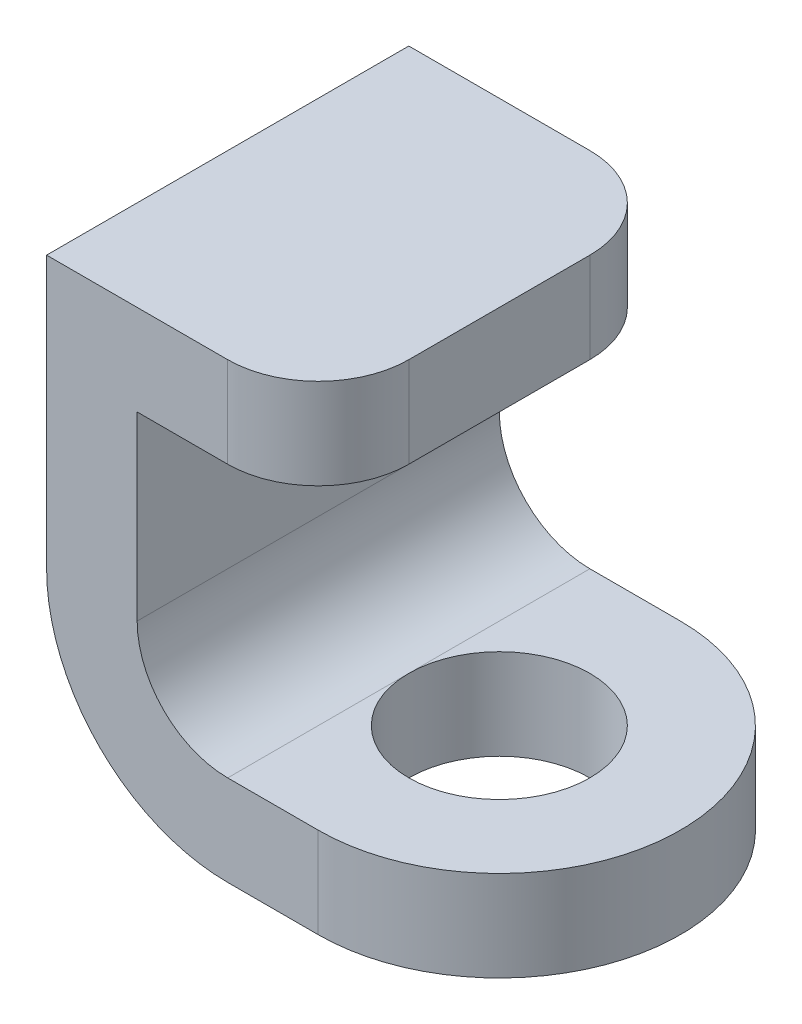
ISO-10303-21;
HEADER;
FILE_DESCRIPTION(('STEP AP214'),'2;1');
FILE_NAME('part.step','',(''),(''),'','','');
FILE_SCHEMA(('AUTOMOTIVE_DESIGN { 1 0 10303 214 1 1 1 1 }'));
ENDSEC;
DATA;
#1=APPLICATION_CONTEXT('core data for automotive mechanical design processes');
#2=APPLICATION_PROTOCOL_DEFINITION('international standard','automotive_design',2000,#1);
#3=PRODUCT_CONTEXT('',#1,'mechanical');
#4=PRODUCT('Part','Part','',(#3));
#5=PRODUCT_RELATED_PRODUCT_CATEGORY('part','',(#4));
#6=PRODUCT_DEFINITION_FORMATION('','',#4);
#7=PRODUCT_DEFINITION_CONTEXT('part definition',#1,'design');
#8=PRODUCT_DEFINITION('design','',#6,#7);
#9=PRODUCT_DEFINITION_SHAPE('','',#8);
#10=(LENGTH_UNIT() NAMED_UNIT(*) SI_UNIT(.MILLI.,.METRE.));
#11=(NAMED_UNIT(*) PLANE_ANGLE_UNIT() SI_UNIT($,.RADIAN.));
#12=(NAMED_UNIT(*) SI_UNIT($,.STERADIAN.) SOLID_ANGLE_UNIT());
#13=UNCERTAINTY_MEASURE_WITH_UNIT(LENGTH_MEASURE(1.E-05),#10,'distance_accuracy_value','');
#14=(GEOMETRIC_REPRESENTATION_CONTEXT(3) GLOBAL_UNCERTAINTY_ASSIGNED_CONTEXT((#13)) GLOBAL_UNIT_ASSIGNED_CONTEXT((#10,
#11,#12)) REPRESENTATION_CONTEXT('',''));
#15=CARTESIAN_POINT('',(0.,0.,0.));
#16=DIRECTION('',(0.,0.,1.));
#17=DIRECTION('',(1.,0.,0.));
#18=AXIS2_PLACEMENT_3D('',#15,#16,#17);
#19=CARTESIAN_POINT('',(50.,0.,20.));
#20=DIRECTION('',(0.,1.,0.));
#21=DIRECTION('',(-1.,0.,0.));
#22=AXIS2_PLACEMENT_3D('',#19,#20,#21);
#23=PLANE('',#22);
#24=DIRECTION('',(0.,0.,-1.));
#25=VECTOR('',#24,1.);
#26=CARTESIAN_POINT('',(20.,0.,20.));
#27=LINE('',#26,#25);
#28=CARTESIAN_POINT('',(20.,0.,20.));
#29=VERTEX_POINT('',#28);
#30=CARTESIAN_POINT('',(20.,0.,0.));
#31=VERTEX_POINT('',#30);
#32=EDGE_CURVE('E215',#29,#31,#27,.T.);
#33=ORIENTED_EDGE('',*,*,#32,.T.);
#34=CARTESIAN_POINT('',(30.,0.,0.));
#35=DIRECTION('',(0.,-1.,0.));
#36=DIRECTION('',(1.,0.,0.));
#37=AXIS2_PLACEMENT_3D('',#34,#35,#36);
#38=CIRCLE('',#37,10.);
#39=EDGE_CURVE('E76',#31,#31,#38,.T.);
#40=ORIENTED_EDGE('',*,*,#39,.F.);
#41=CARTESIAN_POINT('',(20.,0.,-20.));
#42=VERTEX_POINT('',#41);
#43=EDGE_CURVE('E179',#31,#42,#27,.T.);
#44=ORIENTED_EDGE('',*,*,#43,.T.);
#45=DIRECTION('',(1.,0.,0.));
#46=VECTOR('',#45,1.);
#47=CARTESIAN_POINT('',(50.,0.,-20.));
#48=LINE('',#47,#46);
#49=CARTESIAN_POINT('',(30.,0.,-20.));
#50=VERTEX_POINT('',#49);
#51=EDGE_CURVE('E171',#42,#50,#48,.T.);
#52=ORIENTED_EDGE('',*,*,#51,.T.);
#53=CARTESIAN_POINT('',(30.,0.,0.));
#54=DIRECTION('',(0.,-1.,0.));
#55=DIRECTION('',(1.,0.,0.));
#56=AXIS2_PLACEMENT_3D('',#53,#54,#55);
#57=CIRCLE('',#56,20.);
#58=CARTESIAN_POINT('',(30.,0.,20.));
#59=VERTEX_POINT('',#58);
#60=EDGE_CURVE('E154',#50,#59,#57,.T.);
#61=ORIENTED_EDGE('',*,*,#60,.T.);
#62=DIRECTION('',(1.,0.,0.));
#63=VECTOR('',#62,1.);
#64=CARTESIAN_POINT('',(50.,0.,20.));
#65=LINE('',#64,#63);
#66=EDGE_CURVE('E272',#29,#59,#65,.T.);
#67=ORIENTED_EDGE('',*,*,#66,.F.);
#68=EDGE_LOOP('',(#33,#40,#44,#52,#61,#67));
#69=FACE_BOUND('',#68,.T.);
#70=ADVANCED_FACE('F62',(#69),#23,.F.);
#71=CARTESIAN_POINT('',(20.,10.,20.));
#72=DIRECTION('',(0.,-1.,0.));
#73=DIRECTION('',(0.,0.,-1.));
#74=AXIS2_PLACEMENT_3D('',#71,#72,#73);
#75=PLANE('',#74);
#76=DIRECTION('',(0.,0.,-1.));
#77=VECTOR('',#76,1.);
#78=CARTESIAN_POINT('',(20.,10.,20.));
#79=LINE('',#78,#77);
#80=CARTESIAN_POINT('',(20.,10.,0.));
#81=VERTEX_POINT('',#80);
#82=CARTESIAN_POINT('',(20.,10.,-20.));
#83=VERTEX_POINT('',#82);
#84=EDGE_CURVE('E208',#81,#83,#79,.T.);
#85=ORIENTED_EDGE('',*,*,#84,.F.);
#86=CARTESIAN_POINT('',(30.,10.,0.));
#87=DIRECTION('',(0.,-1.,0.));
#88=DIRECTION('',(0.,0.,-1.));
#89=AXIS2_PLACEMENT_3D('',#86,#87,#88);
#90=CIRCLE('',#89,10.);
#91=EDGE_CURVE('E82',#81,#81,#90,.F.);
#92=ORIENTED_EDGE('',*,*,#91,.F.);
#93=CARTESIAN_POINT('',(20.,10.,20.));
#94=VERTEX_POINT('',#93);
#95=EDGE_CURVE('E207',#94,#81,#79,.T.);
#96=ORIENTED_EDGE('',*,*,#95,.F.);
#97=DIRECTION('',(-1.,0.,0.));
#98=VECTOR('',#97,1.);
#99=CARTESIAN_POINT('',(20.,10.,20.));
#100=LINE('',#99,#98);
#101=CARTESIAN_POINT('',(30.,10.,20.));
#102=VERTEX_POINT('',#101);
#103=EDGE_CURVE('E271',#102,#94,#100,.T.);
#104=ORIENTED_EDGE('',*,*,#103,.F.);
#105=CARTESIAN_POINT('',(30.,10.,0.));
#106=DIRECTION('',(0.,-1.,0.));
#107=DIRECTION('',(0.,0.,-1.));
#108=AXIS2_PLACEMENT_3D('',#105,#106,#107);
#109=CIRCLE('',#108,20.);
#110=CARTESIAN_POINT('',(30.,10.,-20.));
#111=VERTEX_POINT('',#110);
#112=EDGE_CURVE('E262',#102,#111,#109,.F.);
#113=ORIENTED_EDGE('',*,*,#112,.T.);
#114=DIRECTION('',(-1.,0.,0.));
#115=VECTOR('',#114,1.);
#116=CARTESIAN_POINT('',(20.,10.,-20.));
#117=LINE('',#116,#115);
#118=EDGE_CURVE('E173',#111,#83,#117,.T.);
#119=ORIENTED_EDGE('',*,*,#118,.T.);
#120=EDGE_LOOP('',(#85,#92,#96,#104,#113,#119));
#121=FACE_BOUND('',#120,.T.);
#122=ADVANCED_FACE('F294',(#121),#75,.F.);
#123=CARTESIAN_POINT('',(0.,50.,20.));
#124=DIRECTION('',(0.,-1.,0.));
#125=DIRECTION('',(0.,0.,-1.));
#126=AXIS2_PLACEMENT_3D('',#123,#124,#125);
#127=PLANE('',#126);
#128=DIRECTION('',(-1.,0.,0.));
#129=VECTOR('',#128,1.);
#130=CARTESIAN_POINT('',(0.,50.,20.));
#131=LINE('',#130,#129);
#132=CARTESIAN_POINT('',(20.,50.,20.));
#133=VERTEX_POINT('',#132);
#134=CARTESIAN_POINT('',(0.,50.,20.));
#135=VERTEX_POINT('',#134);
#136=EDGE_CURVE('E191',#133,#135,#131,.T.);
#137=ORIENTED_EDGE('',*,*,#136,.F.);
#138=CARTESIAN_POINT('',(20.,50.,10.));
#139=DIRECTION('',(0.,-1.,0.));
#140=DIRECTION('',(0.,0.,-1.));
#141=AXIS2_PLACEMENT_3D('',#138,#139,#140);
#142=CIRCLE('',#141,10.);
#143=CARTESIAN_POINT('',(30.,50.,10.));
#144=VERTEX_POINT('',#143);
#145=EDGE_CURVE('E223',#133,#144,#142,.F.);
#146=ORIENTED_EDGE('',*,*,#145,.T.);
#147=DIRECTION('',(0.,0.,-1.));
#148=VECTOR('',#147,1.);
#149=CARTESIAN_POINT('',(30.,50.,20.));
#150=LINE('',#149,#148);
#151=CARTESIAN_POINT('',(30.,50.,-10.));
#152=VERTEX_POINT('',#151);
#153=EDGE_CURVE('E193',#144,#152,#150,.T.);
#154=ORIENTED_EDGE('',*,*,#153,.T.);
#155=CARTESIAN_POINT('',(20.,50.,-10.));
#156=DIRECTION('',(0.,-1.,0.));
#157=DIRECTION('',(0.,0.,-1.));
#158=AXIS2_PLACEMENT_3D('',#155,#156,#157);
#159=CIRCLE('',#158,10.);
#160=CARTESIAN_POINT('',(20.,50.,-20.));
#161=VERTEX_POINT('',#160);
#162=EDGE_CURVE('E224',#152,#161,#159,.F.);
#163=ORIENTED_EDGE('',*,*,#162,.T.);
#164=DIRECTION('',(-1.,0.,0.));
#165=VECTOR('',#164,1.);
#166=CARTESIAN_POINT('',(0.,50.,-20.));
#167=LINE('',#166,#165);
#168=CARTESIAN_POINT('',(0.,50.,-20.));
#169=VERTEX_POINT('',#168);
#170=EDGE_CURVE('E261',#161,#169,#167,.T.);
#171=ORIENTED_EDGE('',*,*,#170,.T.);
#172=DIRECTION('',(0.,0.,-1.));
#173=VECTOR('',#172,1.);
#174=CARTESIAN_POINT('',(0.,50.,20.));
#175=LINE('',#174,#173);
#176=EDGE_CURVE('E220',#135,#169,#175,.T.);
#177=ORIENTED_EDGE('',*,*,#176,.F.);
#178=EDGE_LOOP('',(#137,#146,#154,#163,#171,#177));
#179=FACE_BOUND('',#178,.T.);
#180=ADVANCED_FACE('F252',(#179),#127,.F.);
#181=CARTESIAN_POINT('',(0.,20.,20.));
#182=DIRECTION('',(1.,0.,0.));
#183=DIRECTION('',(0.,1.,0.));
#184=AXIS2_PLACEMENT_3D('',#181,#182,#183);
#185=PLANE('',#184);
#186=DIRECTION('',(0.,-1.,0.));
#187=VECTOR('',#186,1.);
#188=CARTESIAN_POINT('',(0.,20.,-20.));
#189=LINE('',#188,#187);
#190=CARTESIAN_POINT('',(0.,20.,-20.));
#191=VERTEX_POINT('',#190);
#192=EDGE_CURVE('E184',#169,#191,#189,.T.);
#193=ORIENTED_EDGE('',*,*,#192,.T.);
#194=DIRECTION('',(0.,0.,-1.));
#195=VECTOR('',#194,1.);
#196=CARTESIAN_POINT('',(0.,20.,20.));
#197=LINE('',#196,#195);
#198=CARTESIAN_POINT('',(0.,20.,20.));
#199=VERTEX_POINT('',#198);
#200=EDGE_CURVE('E212',#199,#191,#197,.T.);
#201=ORIENTED_EDGE('',*,*,#200,.F.);
#202=DIRECTION('',(0.,-1.,0.));
#203=VECTOR('',#202,1.);
#204=CARTESIAN_POINT('',(0.,20.,20.));
#205=LINE('',#204,#203);
#206=EDGE_CURVE('E280',#135,#199,#205,.T.);
#207=ORIENTED_EDGE('',*,*,#206,.F.);
#208=ORIENTED_EDGE('',*,*,#176,.T.);
#209=EDGE_LOOP('',(#193,#201,#207,#208));
#210=FACE_BOUND('',#209,.T.);
#211=ADVANCED_FACE('F284',(#210),#185,.F.);
#212=CARTESIAN_POINT('',(20.,20.,20.));
#213=DIRECTION('',(0.,0.,-1.));
#214=DIRECTION('',(-1.,0.,0.));
#215=AXIS2_PLACEMENT_3D('',#212,#213,#214);
#216=CYLINDRICAL_SURFACE('',#215,20.);
#217=CARTESIAN_POINT('',(20.,20.,-20.));
#218=DIRECTION('',(0.,0.,1.));
#219=DIRECTION('',(1.,0.,0.));
#220=AXIS2_PLACEMENT_3D('',#217,#218,#219);
#221=CIRCLE('',#220,20.);
#222=EDGE_CURVE('E178',#191,#42,#221,.T.);
#223=ORIENTED_EDGE('',*,*,#222,.T.);
#224=ORIENTED_EDGE('',*,*,#43,.F.);
#225=ORIENTED_EDGE('',*,*,#32,.F.);
#226=CARTESIAN_POINT('',(20.,20.,20.));
#227=DIRECTION('',(0.,0.,1.));
#228=DIRECTION('',(1.,0.,0.));
#229=AXIS2_PLACEMENT_3D('',#226,#227,#228);
#230=CIRCLE('',#229,20.);
#231=EDGE_CURVE('E274',#199,#29,#230,.T.);
#232=ORIENTED_EDGE('',*,*,#231,.F.);
#233=ORIENTED_EDGE('',*,*,#200,.T.);
#234=EDGE_LOOP('',(#223,#224,#225,#232,#233));
#235=FACE_BOUND('',#234,.T.);
#236=ADVANCED_FACE('F286',(#235),#216,.T.);
#237=CARTESIAN_POINT('',(20.,20.,20.));
#238=DIRECTION('',(0.,0.,-1.));
#239=DIRECTION('',(-1.,0.,0.));
#240=AXIS2_PLACEMENT_3D('',#237,#238,#239);
#241=CYLINDRICAL_SURFACE('',#240,10.);
#242=CARTESIAN_POINT('',(20.,20.,-20.));
#243=DIRECTION('',(0.,0.,-1.));
#244=DIRECTION('',(1.,0.,0.));
#245=AXIS2_PLACEMENT_3D('',#242,#243,#244);
#246=CIRCLE('',#245,10.);
#247=CARTESIAN_POINT('',(10.,20.,-20.));
#248=VERTEX_POINT('',#247);
#249=EDGE_CURVE('E185',#83,#248,#246,.T.);
#250=ORIENTED_EDGE('',*,*,#249,.T.);
#251=DIRECTION('',(0.,0.,-1.));
#252=VECTOR('',#251,1.);
#253=CARTESIAN_POINT('',(10.,20.,20.));
#254=LINE('',#253,#252);
#255=CARTESIAN_POINT('',(10.,20.,20.));
#256=VERTEX_POINT('',#255);
#257=EDGE_CURVE('E202',#256,#248,#254,.T.);
#258=ORIENTED_EDGE('',*,*,#257,.F.);
#259=CARTESIAN_POINT('',(20.,20.,20.));
#260=DIRECTION('',(0.,0.,-1.));
#261=DIRECTION('',(1.,0.,0.));
#262=AXIS2_PLACEMENT_3D('',#259,#260,#261);
#263=CIRCLE('',#262,10.);
#264=EDGE_CURVE('E267',#94,#256,#263,.T.);
#265=ORIENTED_EDGE('',*,*,#264,.F.);
#266=ORIENTED_EDGE('',*,*,#95,.T.);
#267=ORIENTED_EDGE('',*,*,#84,.T.);
#268=EDGE_LOOP('',(#250,#258,#265,#266,#267));
#269=FACE_BOUND('',#268,.T.);
#270=ADVANCED_FACE('F297',(#269),#241,.F.);
#271=CARTESIAN_POINT('',(10.,40.,20.));
#272=DIRECTION('',(-1.,0.,0.));
#273=DIRECTION('',(0.,-1.,0.));
#274=AXIS2_PLACEMENT_3D('',#271,#272,#273);
#275=PLANE('',#274);
#276=DIRECTION('',(0.,1.,0.));
#277=VECTOR('',#276,1.);
#278=CARTESIAN_POINT('',(10.,40.,-20.));
#279=LINE('',#278,#277);
#280=CARTESIAN_POINT('',(10.,40.,-20.));
#281=VERTEX_POINT('',#280);
#282=EDGE_CURVE('E188',#248,#281,#279,.T.);
#283=ORIENTED_EDGE('',*,*,#282,.T.);
#284=DIRECTION('',(0.,0.,-1.));
#285=VECTOR('',#284,1.);
#286=CARTESIAN_POINT('',(10.,40.,20.));
#287=LINE('',#286,#285);
#288=CARTESIAN_POINT('',(10.,40.,20.));
#289=VERTEX_POINT('',#288);
#290=EDGE_CURVE('E205',#289,#281,#287,.T.);
#291=ORIENTED_EDGE('',*,*,#290,.F.);
#292=DIRECTION('',(0.,1.,0.));
#293=VECTOR('',#292,1.);
#294=CARTESIAN_POINT('',(10.,40.,20.));
#295=LINE('',#294,#293);
#296=EDGE_CURVE('E247',#256,#289,#295,.T.);
#297=ORIENTED_EDGE('',*,*,#296,.F.);
#298=ORIENTED_EDGE('',*,*,#257,.T.);
#299=EDGE_LOOP('',(#283,#291,#297,#298));
#300=FACE_BOUND('',#299,.T.);
#301=ADVANCED_FACE('F302',(#300),#275,.F.);
#302=CARTESIAN_POINT('',(30.,40.,20.));
#303=DIRECTION('',(0.,1.,0.));
#304=DIRECTION('',(0.,0.,1.));
#305=AXIS2_PLACEMENT_3D('',#302,#303,#304);
#306=PLANE('',#305);
#307=DIRECTION('',(0.,0.,-1.));
#308=VECTOR('',#307,1.);
#309=CARTESIAN_POINT('',(30.,40.,20.));
#310=LINE('',#309,#308);
#311=CARTESIAN_POINT('',(30.,40.,10.));
#312=VERTEX_POINT('',#311);
#313=CARTESIAN_POINT('',(30.,40.,-10.));
#314=VERTEX_POINT('',#313);
#315=EDGE_CURVE('E196',#312,#314,#310,.T.);
#316=ORIENTED_EDGE('',*,*,#315,.F.);
#317=CARTESIAN_POINT('',(20.,40.,10.));
#318=DIRECTION('',(0.,1.,0.));
#319=DIRECTION('',(0.,0.,1.));
#320=AXIS2_PLACEMENT_3D('',#317,#318,#319);
#321=CIRCLE('',#320,10.);
#322=CARTESIAN_POINT('',(20.,40.,20.));
#323=VERTEX_POINT('',#322);
#324=EDGE_CURVE('E72',#312,#323,#321,.F.);
#325=ORIENTED_EDGE('',*,*,#324,.T.);
#326=DIRECTION('',(1.,0.,0.));
#327=VECTOR('',#326,1.);
#328=CARTESIAN_POINT('',(30.,40.,20.));
#329=LINE('',#328,#327);
#330=EDGE_CURVE('E200',#289,#323,#329,.T.);
#331=ORIENTED_EDGE('',*,*,#330,.F.);
#332=ORIENTED_EDGE('',*,*,#290,.T.);
#333=DIRECTION('',(1.,0.,0.));
#334=VECTOR('',#333,1.);
#335=CARTESIAN_POINT('',(30.,40.,-20.));
#336=LINE('',#335,#334);
#337=CARTESIAN_POINT('',(20.,40.,-20.));
#338=VERTEX_POINT('',#337);
#339=EDGE_CURVE('E192',#281,#338,#336,.T.);
#340=ORIENTED_EDGE('',*,*,#339,.T.);
#341=CARTESIAN_POINT('',(20.,40.,-10.));
#342=DIRECTION('',(0.,1.,0.));
#343=DIRECTION('',(0.,0.,1.));
#344=AXIS2_PLACEMENT_3D('',#341,#342,#343);
#345=CIRCLE('',#344,10.);
#346=EDGE_CURVE('E235',#338,#314,#345,.F.);
#347=ORIENTED_EDGE('',*,*,#346,.T.);
#348=EDGE_LOOP('',(#316,#325,#331,#332,#340,#347));
#349=FACE_BOUND('',#348,.T.);
#350=ADVANCED_FACE('F236',(#349),#306,.F.);
#351=CARTESIAN_POINT('',(30.,50.,20.));
#352=DIRECTION('',(-1.,0.,0.));
#353=DIRECTION('',(0.,0.,1.));
#354=AXIS2_PLACEMENT_3D('',#351,#352,#353);
#355=PLANE('',#354);
#356=ORIENTED_EDGE('',*,*,#153,.F.);
#357=DIRECTION('',(0.,1.,0.));
#358=VECTOR('',#357,1.);
#359=CARTESIAN_POINT('',(30.,40.,10.));
#360=LINE('',#359,#358);
#361=EDGE_CURVE('E229',#144,#312,#360,.F.);
#362=ORIENTED_EDGE('',*,*,#361,.T.);
#363=ORIENTED_EDGE('',*,*,#315,.T.);
#364=DIRECTION('',(0.,1.,0.));
#365=VECTOR('',#364,1.);
#366=CARTESIAN_POINT('',(30.,50.,-10.));
#367=LINE('',#366,#365);
#368=EDGE_CURVE('E230',#314,#152,#367,.T.);
#369=ORIENTED_EDGE('',*,*,#368,.T.);
#370=EDGE_LOOP('',(#356,#362,#363,#369));
#371=FACE_BOUND('',#370,.T.);
#372=ADVANCED_FACE('F254',(#371),#355,.F.);
#373=CARTESIAN_POINT('',(20.,20.,20.));
#374=DIRECTION('',(0.,0.,1.));
#375=DIRECTION('',(1.,0.,0.));
#376=AXIS2_PLACEMENT_3D('',#373,#374,#375);
#377=PLANE('',#376);
#378=DIRECTION('',(0.,-1.,0.));
#379=VECTOR('',#378,1.);
#380=CARTESIAN_POINT('',(30.,38.2842712474619,20.));
#381=LINE('',#380,#379);
#382=EDGE_CURVE('E161',#102,#59,#381,.T.);
#383=ORIENTED_EDGE('',*,*,#382,.F.);
#384=ORIENTED_EDGE('',*,*,#103,.T.);
#385=ORIENTED_EDGE('',*,*,#264,.T.);
#386=ORIENTED_EDGE('',*,*,#296,.T.);
#387=ORIENTED_EDGE('',*,*,#330,.T.);
#388=DIRECTION('',(0.,1.,0.));
#389=VECTOR('',#388,1.);
#390=CARTESIAN_POINT('',(20.,50.,20.));
#391=LINE('',#390,#389);
#392=EDGE_CURVE('E219',#323,#133,#391,.T.);
#393=ORIENTED_EDGE('',*,*,#392,.T.);
#394=ORIENTED_EDGE('',*,*,#136,.T.);
#395=ORIENTED_EDGE('',*,*,#206,.T.);
#396=ORIENTED_EDGE('',*,*,#231,.T.);
#397=ORIENTED_EDGE('',*,*,#66,.T.);
#398=EDGE_LOOP('',(#383,#384,#385,#386,#387,#393,#394,#395,#396,#397));
#399=FACE_BOUND('',#398,.T.);
#400=ADVANCED_FACE('F242',(#399),#377,.T.);
#401=CARTESIAN_POINT('',(20.,20.,-20.));
#402=DIRECTION('',(0.,0.,1.));
#403=DIRECTION('',(1.,0.,0.));
#404=AXIS2_PLACEMENT_3D('',#401,#402,#403);
#405=PLANE('',#404);
#406=ORIENTED_EDGE('',*,*,#118,.F.);
#407=DIRECTION('',(0.,-1.,0.));
#408=VECTOR('',#407,1.);
#409=CARTESIAN_POINT('',(30.,38.2842712474619,-20.));
#410=LINE('',#409,#408);
#411=EDGE_CURVE('E158',#111,#50,#410,.T.);
#412=ORIENTED_EDGE('',*,*,#411,.T.);
#413=ORIENTED_EDGE('',*,*,#51,.F.);
#414=ORIENTED_EDGE('',*,*,#222,.F.);
#415=ORIENTED_EDGE('',*,*,#192,.F.);
#416=ORIENTED_EDGE('',*,*,#170,.F.);
#417=DIRECTION('',(0.,1.,0.));
#418=VECTOR('',#417,1.);
#419=CARTESIAN_POINT('',(20.,20.,-20.));
#420=LINE('',#419,#418);
#421=EDGE_CURVE('E12',#161,#338,#420,.F.);
#422=ORIENTED_EDGE('',*,*,#421,.T.);
#423=ORIENTED_EDGE('',*,*,#339,.F.);
#424=ORIENTED_EDGE('',*,*,#282,.F.);
#425=ORIENTED_EDGE('',*,*,#249,.F.);
#426=EDGE_LOOP('',(#406,#412,#413,#414,#415,#416,#422,#423,#424,#425));
#427=FACE_BOUND('',#426,.T.);
#428=ADVANCED_FACE('F166',(#427),#405,.F.);
#429=CARTESIAN_POINT('',(20.,20.,10.));
#430=DIRECTION('',(0.,-1.,0.));
#431=DIRECTION('',(0.,0.,-1.));
#432=AXIS2_PLACEMENT_3D('',#429,#430,#431);
#433=CYLINDRICAL_SURFACE('',#432,10.);
#434=ORIENTED_EDGE('',*,*,#324,.F.);
#435=ORIENTED_EDGE('',*,*,#361,.F.);
#436=ORIENTED_EDGE('',*,*,#145,.F.);
#437=ORIENTED_EDGE('',*,*,#392,.F.);
#438=EDGE_LOOP('',(#434,#435,#436,#437));
#439=FACE_BOUND('',#438,.T.);
#440=ADVANCED_FACE('F246',(#439),#433,.T.);
#441=CARTESIAN_POINT('',(20.,50.,-10.));
#442=DIRECTION('',(0.,1.,0.));
#443=DIRECTION('',(0.,0.,1.));
#444=AXIS2_PLACEMENT_3D('',#441,#442,#443);
#445=CYLINDRICAL_SURFACE('',#444,10.);
#446=ORIENTED_EDGE('',*,*,#346,.F.);
#447=ORIENTED_EDGE('',*,*,#421,.F.);
#448=ORIENTED_EDGE('',*,*,#162,.F.);
#449=ORIENTED_EDGE('',*,*,#368,.F.);
#450=EDGE_LOOP('',(#446,#447,#448,#449));
#451=FACE_BOUND('',#450,.T.);
#452=ADVANCED_FACE('F64',(#451),#445,.T.);
#453=CARTESIAN_POINT('',(30.,38.2842712474619,0.));
#454=DIRECTION('',(0.,-1.,0.));
#455=DIRECTION('',(1.,0.,0.));
#456=AXIS2_PLACEMENT_3D('',#453,#454,#455);
#457=CYLINDRICAL_SURFACE('',#456,20.);
#458=ORIENTED_EDGE('',*,*,#382,.T.);
#459=ORIENTED_EDGE('',*,*,#60,.F.);
#460=ORIENTED_EDGE('',*,*,#411,.F.);
#461=ORIENTED_EDGE('',*,*,#112,.F.);
#462=EDGE_LOOP('',(#458,#459,#460,#461));
#463=FACE_BOUND('',#462,.T.);
#464=ADVANCED_FACE('F160',(#463),#457,.T.);
#465=CARTESIAN_POINT('',(30.,38.2842712474619,0.));
#466=DIRECTION('',(0.,-1.,0.));
#467=DIRECTION('',(1.,0.,0.));
#468=AXIS2_PLACEMENT_3D('',#465,#466,#467);
#469=CYLINDRICAL_SURFACE('',#468,10.);
#470=ORIENTED_EDGE('',*,*,#91,.T.);
#471=EDGE_LOOP('',(#470));
#472=FACE_BOUND('',#471,.T.);
#473=ORIENTED_EDGE('',*,*,#39,.T.);
#474=EDGE_LOOP('',(#473));
#475=FACE_BOUND('',#474,.T.);
#476=ADVANCED_FACE('F410',(#472,#475),#469,.F.);
#477=CLOSED_SHELL('',(#70,#122,#180,#211,#236,#270,#301,#350,#372,#400,#428,#440,#452,#464,#476));
#478=MANIFOLD_SOLID_BREP('B2',#477);
#479=ADVANCED_BREP_SHAPE_REPRESENTATION('',(#18,#478),#14);
#480=SHAPE_DEFINITION_REPRESENTATION(#9,#479);
ENDSEC;
END-ISO-10303-21;
